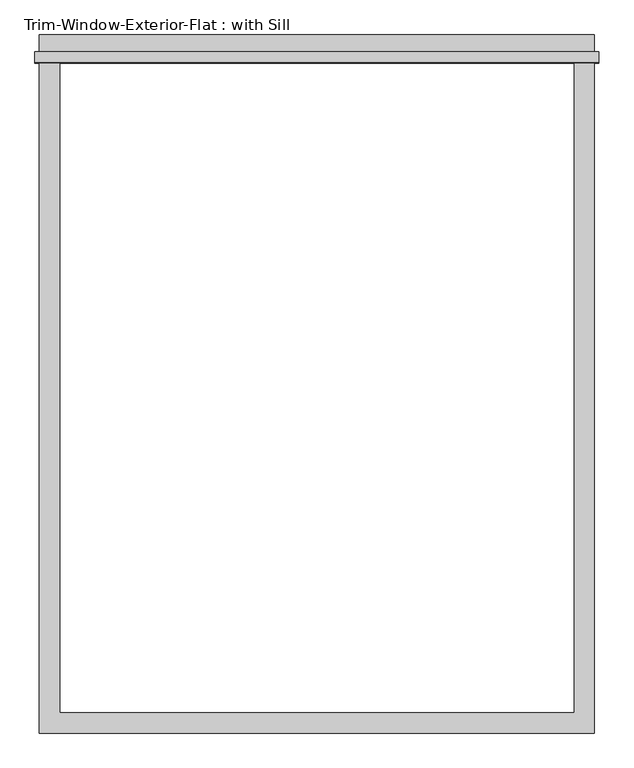
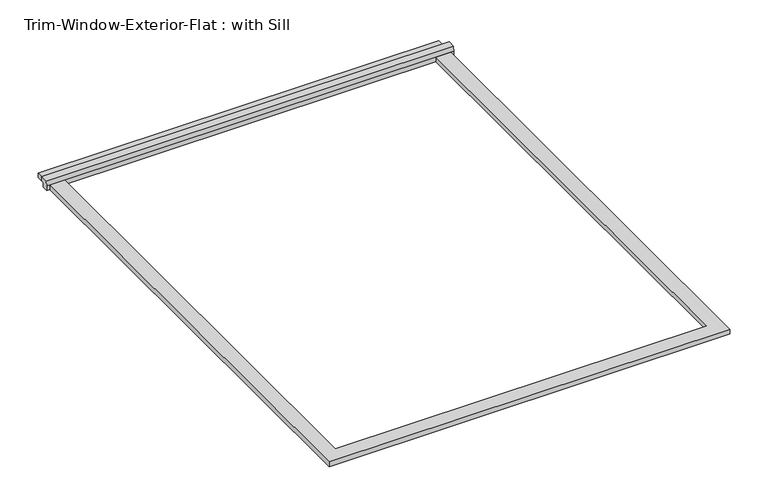
"""IFC4 building model written with IfcOpenShell, lengths in millimetres: proxy geometry, Trim-Window-Exterior-Flat : with Sill."""

from ifc_helpers import new_model, si_unit, frame, origin, origin_with_axes, place, context, project, spatial, polyline, outline, extrude, source, transform, mapped, element, save


def trim_window_exterior_flat_with_sill_a4fd29d2(model_context):
    return source(origin(), model_context, "Body", "SweptSolid", [
        extrude(outline(polyline([(781.05, 1850.9823709), (-781.05, 1850.9823709), (-781.05, 1908.1323709), (781.05, 1908.1323709), (781.05, 1850.9823709)])), origin_with_axes(), (0.0, 0.0, 1.0), 19.05),
        extrude(outline(polyline([(1860.55, 38.1), (1860.55, 19.05), (1850.9823709, 19.05), (1850.9823709, 0.0), (1828.8, 0.0), (1828.8, 19.05), (1831.2580645, 38.1), (1860.55, 38.1)])), frame((-793.75, 0.0, 0.0), z_axis=(1.0, 0.0, 0.0), x_axis=(0.0, 1.0, 0.0)), (0.0, 0.0, 1.0), 1587.5),
        extrude(outline(polyline([(-781.05, -57.15), (-781.05, 1828.8), (-723.9, 1828.8), (-723.9, 0.0), (723.9, 0.0), (723.9, 1828.8), (781.05, 1828.8), (781.05, -57.15), (-781.05, -57.15)])), origin_with_axes(), (0.0, 0.0, 1.0), 19.05),
    ])


if __name__ == "__main__":
    model = new_model("IFC4")
    model_context = context("Model", 3, world=origin())
    ifc_project = project(units=[si_unit("LENGTHUNIT", "METRE", prefix="MILLI")], contexts=[model_context])
    site = spatial("IfcSite", under=ifc_project)
    building = spatial("IfcBuilding", under=site)
    placement = place(None, origin())
    trim_window_exterior_flat_with_sill_shape = trim_window_exterior_flat_with_sill_a4fd29d2(model_context)
    element("IfcBuildingElementProxy", 1, Name="Trim-Window-Exterior-Flat : with Sill", ObjectType="Trim-Window-Exterior-Flat : with Sill", at=placement, inside=building, context=model_context, shape_type="MappedRepresentation", body=[
        mapped(trim_window_exterior_flat_with_sill_shape, transform((0.0, 0.0, 0.0), x_axis=(1.0, 0.0, 0.0), y_axis=(0.0, 1.0, 0.0), z_axis=(0.0, 0.0, 1.0))),
    ])
    save(model, "model.ifc")

# Revit data of these elements
# Type "Trim-Window-Exterior-Flat : with Sill"
#   Trim Width = 0' - 2 1/4"
#   Trim Thickness_Picture Frame = 0' - 1 1/4"
#   Trim Thickness_with Sill = 0' - 0 3/4"
#   Sill Thickness = 0' - 1 1/4"
#   Opening Width [instance default] = 2' - 0"
#   Opening Height [instance default] = 3' - 0"
#   Default Elevation = 4' - 0"
#   Sill = yes
#   Picture Frame = no
#   Trim Material [instance default] = none
# Element 1 (IfcBuildingElementProxy, "Trim-Window-Exterior-Flat : with Sill")
#   Opening Width = 4' - 9"
#   Opening Height = 6' - 0"
#   Trim Material = Clad - White
#   Materials on its faces: "Clad - White"
# Materials
#   "Clad - White": class "Wood", colour RGB 242 242 238, transparency 0, Cost = 0
